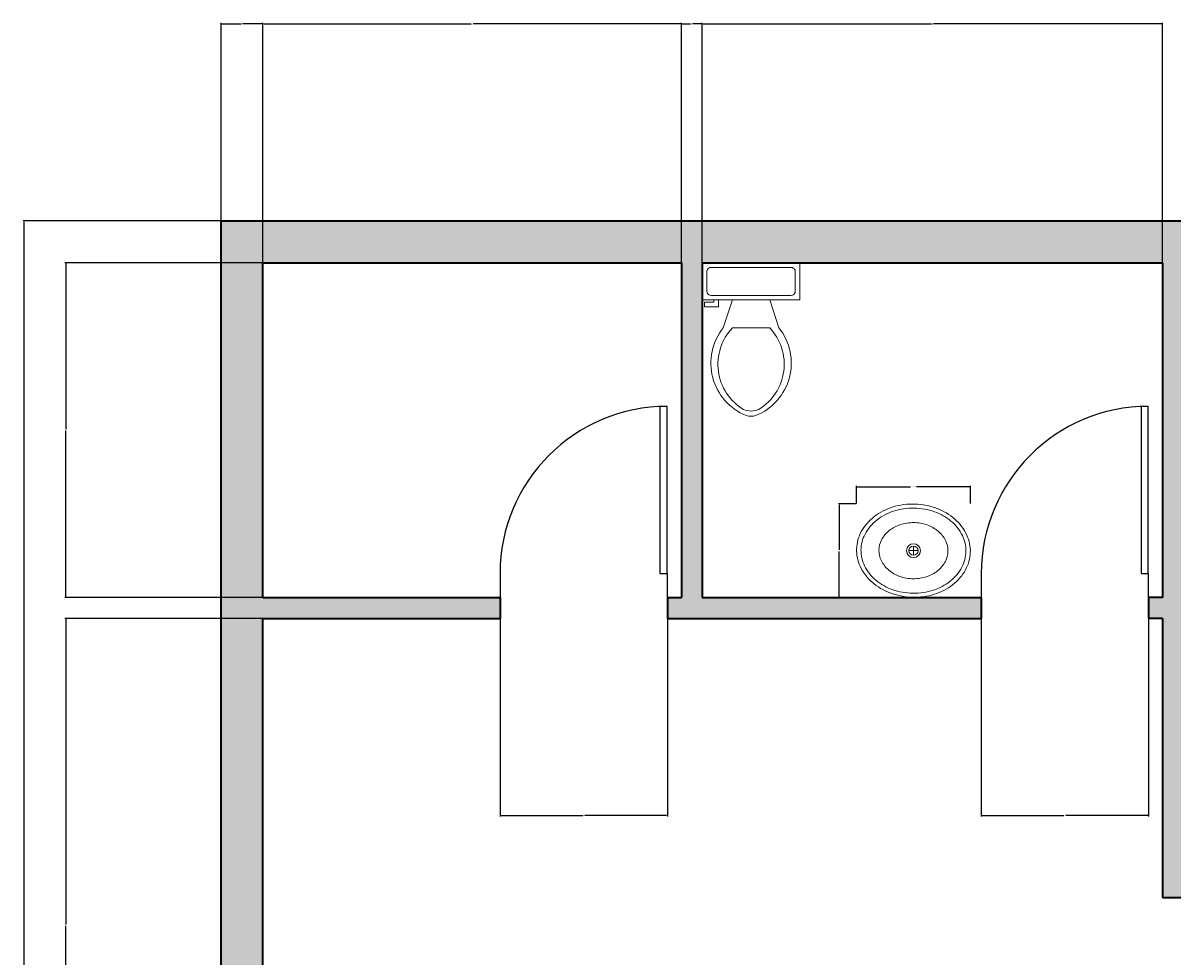
# Model space of a CAD drawing. Units: inches. Extents: x 1563 to 2428, y 777 to 1464.
# Tile 6 of 11: x 1563 to 1810, y 1263 to 1464. Entities that reach past the tile are written whole.
import ezdxf

# ---------------------------------------------------------------- set-up
doc = ezdxf.new("R2010")
doc.units = ezdxf.units.IN
for name, color, linetype, lineweight in [('A-ANNO-DIMS', 2, 'Continuous', 18), ('A-DOOR', 4, 'Continuous', 25), ('A-FLOR-FIXT', 9, 'Continuous', 20), ('A-WALL', 7, 'Continuous', 35), ('A-WALL-PATT', 8, 'Continuous', 13)]:
    doc.layers.add(name, color=color, linetype=linetype, lineweight=lineweight)
doc.styles.get("Standard").update_dxf_attribs({"font": 'arial.ttf'})
doc.dimstyles.get("Standard").update_dxf_attribs({"dimtxt": 0.18, "dimasz": 0.18, "dimexe": 0.18, "dimexo": 0.0625, "dimgap": 0.09, "dimtad": 0, "dimtih": 1, "dimtoh": 1, "dimdec": 4, "dimzin": 0, "dimdsep": 46, "dimtxsty": 'Standard', "dimcen": 0.09, "dimadec": 0, "dimazin": 0, "dimtfac": 1, "dimtdec": 4, "dimtofl": 0, "dimtmove": 0, "dimatfit": 3, "dimfxl": 1, "dimtolj": 1, "dimtzin": 0, "dimarcsym": 0})

# ---------------------------------------------------------------- blocks, each defined once
blk = doc.blocks.new('*U3')
for p, q in [((0, 0), (0, -6)), ((-40, 0), (-40, -6))]:
    blk.add_line(p, q)
blk.add_lwpolyline([(0, 0), (0, 40), (-1.75, 40), (-1.75, 0)], close=True)
blk.add_arc((0, 0), 40, 90, 180)
blk = doc.blocks.new('Toilet - top')
for p, q in [((9.5, -6), (9.5, -2)), ((-10, -8.5), (-8, -8.5)), ((-10, -9.5), (-10, -8.5)), ((-7, -9.5), (-10, -9.5)), ((-8, -8.5), (-8, -8)), ((-7, -8), (-7, -9.5)), ((-4, -8), (-6, -14)), ((4, -8), (6, -14)), ((4, -14), (-4, -14))]:
    blk.add_line(p, q)
blk.add_lwpolyline([(10.5, -8), (10.5, 0), (-10.5, 0), (-10.5, -8)], close=True)
for points in [[(-9.5, -2), (-9.5, -6)], [(8.5, -1), (-8.5, -1)], [(-8.5, -7), (8.5, -7)]]:
    blk.add_lwpolyline(points)
for centre, radius, start, end in [((-8.62, -1.88), 0.884, 81.8699, 188.1301), ((8.62, -1.88), 0.884, 351.8699, 98.1301), ((-8.62, -6.12), 0.884, 171.8699, 278.1301), ((8.62, -6.12), 0.884, 261.8699, 8.1301), ((3.52, -21.58), 12.17, 141.4691, 247.9714), ((4.2, -21.82), 11.33, 136.3677, 238.9468), ((-3.52, -21.58), 12.17, 292.0284, 38.5307), ((-4.2, -21.82), 11.33, 301.053, 43.6321), ((0, -27.88), 4, 245.7318, 294.2682), ((0, -29), 4, 254.8605, 285.1395)]:
    blk.add_arc(centre, radius, start, end)
blk = doc.blocks.new('Sink - Oval top')
for p, q in [((-1, 0), (1, 0)), ((0, 1), (0, -1))]:
    blk.add_line(p, q)
for points in [[(-12.23, 0.39, 0.117634), (-11.46, -3.36, 0.104469), (-8.88, -6.8, 0.090016), (-5.08, -9.07, 0.08192), (-0.32, -10.02, 0.08192), (4.49, -9.38, 0.090016), (8.42, -7.36, 0.104469), (11.22, -4.09, 0.117634), (12.23, -0.39, 0.117634), (11.46, 3.36, 0.104469), (8.88, 6.8, 0.090016), (5.08, 9.07, 0.08192), (0.32, 10.02, 0.08192), (-4.49, 9.38, 0.090016), (-8.42, 7.36, 0.104469), (-11.22, 4.09, 0.117634)], [(-11.29, 0.16, 0.118622), (-10.52, -3.25, 0.104678), (-8.07, -6.36, 0.089562), (-4.54, -8.37, 0.081185), (-0.13, -9.15, 0.081185), (4.3, -8.49, 0.089562), (7.89, -6.58, 0.104678), (10.42, -3.55, 0.118622), (11.29, -0.16, 0.118622), (10.52, 3.25, 0.104678), (8.07, 6.36, 0.089562), (4.54, 8.37, 0.081185), (0.13, 9.15, 0.081185), (-4.3, 8.49, 0.089562), (-7.89, 6.58, 0.104678), (-10.42, 3.55, 0.118622)], [(-7.42, 0.08, 0.118283), (-6.91, -2.17, 0.104607), (-5.29, -4.21, 0.089718), (-2.97, -5.53, 0.081436), (-0.07, -6.04, 0.081436), (2.84, -5.59, 0.089718), (5.2, -4.33, 0.104607), (6.86, -2.32, 0.118283), (7.42, -0.08, 0.118283), (6.91, 2.17, 0.104607), (5.29, 4.21, 0.089718), (2.97, 5.53, 0.081436), (0.07, 6.04, 0.081436), (-2.84, 5.59, 0.089718), (-5.2, 4.33, 0.104607), (-6.86, 2.32, 0.118283)]]:
    blk.add_lwpolyline(points, format="xyb", close=True)
for radius in [1.5, 1]:
    blk.add_circle((0, 0), radius)
blk = doc.blocks.new('*D44')
at = {"layer": 'A-ANNO-DIMS', "color": 0, "lineweight": -2, "transparency": 16777216}
for p, q in [((1741.76, 1360.64), (1741.76, 1364.44)), ((1741.94, 1364.26), (1753.4, 1364.26)), ((1766.13, 1364.26), (1754.66, 1364.26)), ((1766.31, 1360.64), (1766.31, 1364.44))]:
    blk.add_line(p, q, dxfattribs=at)
at = {"layer": 'A-ANNO-DIMS', "color": 0, "transparency": 16777216}
for points in [[(1741.94, 1364.29), (1741.94, 1364.23), (1741.76, 1364.26)], [(1766.13, 1364.29), (1766.13, 1364.23), (1766.31, 1364.26)]]:
    blk.add_solid(points, dxfattribs=at)
at = {"layer": 'Defpoints', "color": 0, "transparency": 16777216}
for p in [(1766.31, 1364.26), (1741.76, 1360.58), (1766.31, 1360.58)]:
    blk.add_point(p, dxfattribs=at)
at = {"layer": 'A-ANNO-DIMS', "color": 0, "transparency": 16777216, "insert": (1754.03, 1364.26), "char_height": 0.18, "attachment_point": 5}
blk.add_mtext('\\A1;BASIN 25', dxfattribs=at)
blk = doc.blocks.new('*D45')
at = {"layer": 'A-ANNO-DIMS', "color": 0, "lineweight": -2, "transparency": 16777216}
for p, q in [((1741.69, 1360.58), (1737.89, 1360.58)), ((1738.07, 1360.4), (1738.07, 1350.69)), ((1738.07, 1340.62), (1738.07, 1350.33)), ((1741.69, 1340.44), (1737.89, 1340.44))]:
    blk.add_line(p, q, dxfattribs=at)
at = {"layer": 'A-ANNO-DIMS', "color": 0, "transparency": 16777216}
for points in [[(1738.04, 1360.4), (1738.1, 1360.4), (1738.07, 1360.58)], [(1738.04, 1340.62), (1738.1, 1340.62), (1738.07, 1340.44)]]:
    blk.add_solid(points, dxfattribs=at)
at = {"layer": 'Defpoints', "color": 0, "transparency": 16777216}
for p in [(1738.07, 1360.58), (1741.76, 1360.58), (1741.76, 1340.44)]:
    blk.add_point(p, dxfattribs=at)
at = {"layer": 'A-ANNO-DIMS', "color": 0, "transparency": 16777216, "insert": (1738.07, 1350.51), "char_height": 0.18, "attachment_point": 5}
blk.add_mtext('\\A1;20', dxfattribs=at)
blk = doc.blocks.new('*D49')
at = {"layer": 'A-ANNO-DIMS', "color": 0, "lineweight": -2, "transparency": 16777216}
for p, q in [((1605.04, 1421.43), (1562.53, 1421.43)), ((1562.71, 1421.25), (1562.71, 1121.61)), ((1562.71, 821.61), (1562.71, 1121.25)), ((1605.04, 821.43), (1562.53, 821.43))]:
    blk.add_line(p, q, dxfattribs=at)
at = {"layer": 'A-ANNO-DIMS', "color": 0, "transparency": 16777216}
for points in [[(1562.68, 1421.25), (1562.74, 1421.25), (1562.71, 1421.43)], [(1562.68, 821.61), (1562.74, 821.61), (1562.71, 821.43)]]:
    blk.add_solid(points, dxfattribs=at)
at = {"layer": 'Defpoints', "color": 0, "transparency": 16777216}
for p in [(1562.71, 1421.43), (1605.11, 1421.43), (1605.11, 821.43)]:
    blk.add_point(p, dxfattribs=at)
at = {"layer": 'A-ANNO-DIMS', "color": 0, "transparency": 16777216, "insert": (1562.71, 1121.43), "char_height": 0.18, "attachment_point": 5}
blk.add_mtext('\\A1;600', dxfattribs=at)
blk = doc.blocks.new('*D50')
at = {"layer": 'A-ANNO-DIMS', "color": 0, "lineweight": -2, "transparency": 16777216}
for p, q in [((1614.11, 1412.49), (1614.11, 1464.01)), ((1614.29, 1463.83), (1658.89, 1463.83)), ((1703.93, 1463.83), (1659.32, 1463.83)), ((1704.11, 1412.49), (1704.11, 1464.01))]:
    blk.add_line(p, q, dxfattribs=at)
at = {"layer": 'A-ANNO-DIMS', "color": 0, "transparency": 16777216}
for points in [[(1614.29, 1463.86), (1614.29, 1463.8), (1614.11, 1463.83)], [(1703.93, 1463.86), (1703.93, 1463.8), (1704.11, 1463.83)]]:
    blk.add_solid(points, dxfattribs=at)
at = {"layer": 'Defpoints', "color": 0, "transparency": 16777216}
for p in [(1704.11, 1463.83), (1614.11, 1412.43), (1704.11, 1412.43)]:
    blk.add_point(p, dxfattribs=at)
at = {"layer": 'A-ANNO-DIMS', "color": 0, "transparency": 16777216, "insert": (1659.11, 1463.83), "char_height": 0.18, "attachment_point": 5}
blk.add_mtext('\\A1;90', dxfattribs=at)
blk = doc.blocks.new('*D51')
at = {"layer": 'A-ANNO-DIMS', "color": 0, "lineweight": -2, "transparency": 16777216}
for p, q in [((1708.61, 1412.49), (1708.61, 1464.01)), ((1708.79, 1463.83), (1757.89, 1463.83)), ((1807.43, 1463.83), (1758.32, 1463.83)), ((1807.61, 1412.49), (1807.61, 1464.01))]:
    blk.add_line(p, q, dxfattribs=at)
at = {"layer": 'A-ANNO-DIMS', "color": 0, "transparency": 16777216}
for points in [[(1708.79, 1463.86), (1708.79, 1463.8), (1708.61, 1463.83)], [(1807.43, 1463.86), (1807.43, 1463.8), (1807.61, 1463.83)]]:
    blk.add_solid(points, dxfattribs=at)
at = {"layer": 'Defpoints', "color": 0, "transparency": 16777216}
for p in [(1807.61, 1463.83), (1708.61, 1412.43), (1807.61, 1412.43)]:
    blk.add_point(p, dxfattribs=at)
at = {"layer": 'A-ANNO-DIMS', "color": 0, "transparency": 16777216, "insert": (1758.11, 1463.83), "char_height": 0.18, "attachment_point": 5}
blk.add_mtext('\\A1;99', dxfattribs=at)
blk = doc.blocks.new('*D53')
at = {"layer": 'A-ANNO-DIMS', "color": 0, "lineweight": -2, "transparency": 16777216}
for p, q in [((1614.04, 1412.43), (1571.53, 1412.43)), ((1571.71, 1412.25), (1571.71, 1376.61)), ((1571.71, 1340.61), (1571.71, 1376.25)), ((1614.04, 1340.43), (1571.53, 1340.43))]:
    blk.add_line(p, q, dxfattribs=at)
at = {"layer": 'A-ANNO-DIMS', "color": 0, "transparency": 16777216}
for points in [[(1571.68, 1412.25), (1571.74, 1412.25), (1571.71, 1412.43)], [(1571.68, 1340.61), (1571.74, 1340.61), (1571.71, 1340.43)]]:
    blk.add_solid(points, dxfattribs=at)
at = {"layer": 'Defpoints', "color": 0, "transparency": 16777216}
for p in [(1571.71, 1412.43), (1614.11, 1412.43), (1614.11, 1340.43)]:
    blk.add_point(p, dxfattribs=at)
at = {"layer": 'A-ANNO-DIMS', "color": 0, "transparency": 16777216, "insert": (1571.71, 1376.43), "char_height": 0.18, "attachment_point": 5}
blk.add_mtext('\\A1;72', dxfattribs=at)
blk = doc.blocks.new('*D55')
at = {"layer": 'A-ANNO-DIMS', "color": 0, "lineweight": -2, "transparency": 16777216}
for p, q in [((1614.04, 1335.93), (1571.53, 1335.93)), ((1571.71, 1335.75), (1571.71, 1270.11)), ((1571.71, 1204.11), (1571.71, 1269.75)), ((1614.04, 1203.93), (1571.53, 1203.93))]:
    blk.add_line(p, q, dxfattribs=at)
at = {"layer": 'A-ANNO-DIMS', "color": 0, "transparency": 16777216}
for points in [[(1571.68, 1335.75), (1571.74, 1335.75), (1571.71, 1335.93)], [(1571.68, 1204.11), (1571.74, 1204.11), (1571.71, 1203.93)]]:
    blk.add_solid(points, dxfattribs=at)
at = {"layer": 'Defpoints', "color": 0, "transparency": 16777216}
for p in [(1571.71, 1335.93), (1614.11, 1335.93), (1614.11, 1203.93)]:
    blk.add_point(p, dxfattribs=at)
at = {"layer": 'A-ANNO-DIMS', "color": 0, "transparency": 16777216, "insert": (1571.71, 1269.93), "char_height": 0.18, "attachment_point": 5}
blk.add_mtext('\\A1;132', dxfattribs=at)
blk = doc.blocks.new('*D65')
at = {"layer": 'A-ANNO-DIMS', "color": 0, "lineweight": -2, "transparency": 16777216}
for p, q in [((1665.11, 1335.87), (1665.11, 1293.35)), ((1701.11, 1335.87), (1701.11, 1293.35)), ((1665.29, 1293.53), (1682.89, 1293.53)), ((1700.93, 1293.53), (1683.32, 1293.53))]:
    blk.add_line(p, q, dxfattribs=at)
at = {"layer": 'A-ANNO-DIMS', "color": 0, "transparency": 16777216}
for points in [[(1665.29, 1293.56), (1665.29, 1293.5), (1665.11, 1293.53)], [(1700.93, 1293.56), (1700.93, 1293.5), (1701.11, 1293.53)]]:
    blk.add_solid(points, dxfattribs=at)
at = {"layer": 'Defpoints', "color": 0, "transparency": 16777216}
for p in [(1665.11, 1335.93), (1701.11, 1335.93), (1665.11, 1293.53)]:
    blk.add_point(p, dxfattribs=at)
at = {"layer": 'A-ANNO-DIMS', "color": 0, "transparency": 16777216, "insert": (1683.11, 1293.53), "char_height": 0.18, "attachment_point": 5}
blk.add_mtext('\\A1;36', dxfattribs=at)
blk = doc.blocks.new('*D66')
at = {"layer": 'A-ANNO-DIMS', "color": 0, "lineweight": -2, "transparency": 16777216}
for p, q in [((1768.61, 1335.87), (1768.61, 1293.35)), ((1804.61, 1335.87), (1804.61, 1293.35)), ((1768.79, 1293.53), (1786.39, 1293.53)), ((1804.43, 1293.53), (1786.82, 1293.53))]:
    blk.add_line(p, q, dxfattribs=at)
at = {"layer": 'A-ANNO-DIMS', "color": 0, "transparency": 16777216}
for points in [[(1768.79, 1293.56), (1768.79, 1293.5), (1768.61, 1293.53)], [(1804.43, 1293.56), (1804.43, 1293.5), (1804.61, 1293.53)]]:
    blk.add_solid(points, dxfattribs=at)
at = {"layer": 'Defpoints', "color": 0, "transparency": 16777216}
for p in [(1768.61, 1335.93), (1804.61, 1335.93), (1768.61, 1293.53)]:
    blk.add_point(p, dxfattribs=at)
at = {"layer": 'A-ANNO-DIMS', "color": 0, "transparency": 16777216, "insert": (1786.61, 1293.53), "char_height": 0.18, "attachment_point": 5}
blk.add_mtext('\\A1;36', dxfattribs=at)
blk = doc.blocks.new('*D71')
at = {"layer": 'A-ANNO-DIMS', "color": 0, "lineweight": -2, "transparency": 16777216}
for p, q in [((1704.11, 1412.49), (1704.11, 1464.01)), ((1704.29, 1463.83), (1706.1, 1463.83)), ((1708.43, 1463.83), (1706.61, 1463.83)), ((1708.61, 1412.49), (1708.61, 1464.01))]:
    blk.add_line(p, q, dxfattribs=at)
at = {"layer": 'A-ANNO-DIMS', "color": 0, "transparency": 16777216}
for points in [[(1704.29, 1463.86), (1704.29, 1463.8), (1704.11, 1463.83)], [(1708.43, 1463.86), (1708.43, 1463.8), (1708.61, 1463.83)]]:
    blk.add_solid(points, dxfattribs=at)
at = {"layer": 'Defpoints', "color": 0, "transparency": 16777216}
for p in [(1708.61, 1463.83), (1704.11, 1412.43), (1708.61, 1412.43)]:
    blk.add_point(p, dxfattribs=at)
at = {"layer": 'A-ANNO-DIMS', "color": 0, "transparency": 16777216, "insert": (1706.36, 1463.83), "char_height": 0.18, "attachment_point": 5}
blk.add_mtext('\\A1;4.5', dxfattribs=at)
blk = doc.blocks.new('*D72')
at = {"layer": 'A-ANNO-DIMS', "color": 0, "lineweight": -2, "transparency": 16777216}
for p, q in [((1605.11, 1421.49), (1605.11, 1464.01)), ((1605.29, 1463.83), (1609.46, 1463.83)), ((1613.93, 1463.83), (1609.75, 1463.83)), ((1614.11, 1412.49), (1614.11, 1464.01))]:
    blk.add_line(p, q, dxfattribs=at)
at = {"layer": 'A-ANNO-DIMS', "color": 0, "transparency": 16777216}
for points in [[(1605.29, 1463.86), (1605.29, 1463.8), (1605.11, 1463.83)], [(1613.93, 1463.86), (1613.93, 1463.8), (1614.11, 1463.83)]]:
    blk.add_solid(points, dxfattribs=at)
at = {"layer": 'Defpoints', "color": 0, "transparency": 16777216}
for p in [(1614.11, 1463.83), (1605.11, 1421.43), (1614.11, 1412.43)]:
    blk.add_point(p, dxfattribs=at)
at = {"layer": 'A-ANNO-DIMS', "color": 0, "transparency": 16777216, "insert": (1609.61, 1463.83), "char_height": 0.18, "attachment_point": 5}
blk.add_mtext('\\A1;9', dxfattribs=at)

msp = doc.modelspace()

# ---------------------------------------------------------------- hatches: boundary and pattern name
at = {"layer": 'A-WALL-PATT'}
h = msp.add_hatch(color=256, dxfattribs=at)
h.dxf.hatch_style = 1
h.paths.add_polyline_path([(1965.105, 1421.428), (1605.105, 1421.428), (1605.105, 821.428), (1965.105, 821.428)])
h.paths.add_polyline_path([(1614.105, 1199.428), (1704.105, 1199.428), (1738.605, 1199.428), (1738.605, 1251.928), (1734.105, 1251.928), (1734.105, 1203.928), (1704.105, 1203.928), (1614.105, 1203.928), (1614.105, 1335.928), (1665.105, 1335.928), (1665.105, 1340.428), (1614.105, 1340.428), (1614.105, 1412.428), (1704.105, 1412.428), (1704.105, 1340.428), (1701.105, 1340.428), (1701.105, 1335.928), (1704.105, 1335.928), (1768.605, 1335.928), (1768.605, 1340.428), (1708.605, 1340.428), (1708.605, 1412.428), (1807.605, 1412.428), (1807.605, 1340.428), (1804.605, 1340.428), (1804.605, 1335.928), (1807.605, 1335.928), (1807.605, 1275.928), (1815.105, 1275.928), (1815.105, 1280.428), (1812.105, 1280.428), (1812.105, 1412.428), (1956.105, 1412.428), (1956.105, 1280.428), (1854.105, 1280.428), (1854.105, 1275.928), (1956.105, 1275.928), (1956.105, 830.428), (1614.105, 830.428)], flags=16)
h.paths.add_polyline_path([(1917.224, 1038.928), (1917.224, 1043.846, -0.4014527), (1951.591, 1079.751), (1951.591, 1079.786), (1953.163, 1079.786), (1953.163, 1043.846), (1953.163, 1038.455), (1953.105, 1034.428), (1953.105, 1038.928), (1953.163, 1043.846), (1951.591, 1043.846), (1951.591, 1079.751, 0.4014527), (1917.224, 1043.846), (1917.224, 1038.455), (1917.224, 1034.428), (1834.605, 1034.428), (1834.605, 906.928), (1858.605, 906.928), (1858.605, 954.928), (1932.105, 954.928), (1932.105, 902.428), (1834.605, 902.428), (1834.605, 1034.428), (1914.224, 1034.428), (1914.224, 1038.928)], flags=0)
edge = h.paths.add_edge_path(flags=0)
edge.add_ellipse((1674.345, 1004.483), major_axis=(1.48, 0), ratio=0.8423039, start_angle=90, end_angle=180, ccw=False)
edge.add_line((1674.345, 1005.73), (1674.921, 1005.73))
edge.add_ellipse((2202.617, 985.642), major_axis=(528.234, 0), ratio=0.8423039, start_angle=176.34957, end_angle=177.82005, ccw=False)
edge.add_ellipse((1739.278, 760.804), major_axis=(-313.308, 0), ratio=0.8423039, start_angle=-77.87403, end_angle=-76.21947, ccw=False)
edge.add_ellipse((1739.278, 767.659), major_axis=(305.303, 0), ratio=0.8423039, start_angle=100.20954, end_angle=102.44463, ccw=False)
edge.add_ellipse((1659.357, 1231.328), major_axis=(250.96, 0), ratio=0.8423039, start_angle=-80.74343, end_angle=-77.44507)
edge.add_line((1705.625, 1023.567), (1711.685, 1026.918))
edge.add_ellipse((1711.754, 1026.21), major_axis=(0.74, 0), ratio=0.8423039, start_angle=52.06687, end_angle=90, ccw=False)
edge.add_line((1712.16, 1026.731), (1717.882, 1023.567))
edge.add_ellipse((1764.151, 1231.328), major_axis=(250.96, 0), ratio=0.8423039, start_angle=257.44507, end_angle=260.74343)
edge.add_ellipse((1684.229, 767.659), major_axis=(305.303, 0), ratio=0.8423039, start_angle=77.55537, end_angle=79.79046, ccw=False)
edge.add_ellipse((1684.229, 760.804), major_axis=(-313.308, 0), ratio=0.8423039, start_angle=256.21947, end_angle=257.87403, ccw=False)
edge.add_ellipse((1220.891, 985.642), major_axis=(-528.234, 0), ratio=0.8423039, start_angle=182.17995, end_angle=183.65043, ccw=False)
edge.add_line((1748.586, 1005.73), (1749.162, 1005.73))
edge.add_ellipse((1749.162, 1004.483), major_axis=(-1.48, 0), ratio=0.8423039, start_angle=180, end_angle=270, ccw=False)
edge.add_line((1750.642, 1004.483), (1750.642, 980.28))
edge.add_ellipse((1749.162, 980.28), major_axis=(1.48, 0), ratio=0.8423039, start_angle=270, end_angle=360, ccw=False)
edge.add_ellipse((-8843.864, 962.352), major_axis=(10593.026, 0), ratio=0.84230387, start_angle=-0.3241203, end_angle=0.0902291, ccw=False)
edge.add_ellipse((-8843.864, 962.352), major_axis=(10593.026, 0), ratio=0.84230387, start_angle=-0.3838668, end_angle=-0.3241203, ccw=False)
edge.add_ellipse((1749.162, 890.136), major_axis=(1.48, 0), ratio=0.8423039, start_angle=0, end_angle=90, ccw=False)
edge.add_line((1750.642, 890.136), (1750.642, 865.933))
edge.add_ellipse((1749.162, 865.933), major_axis=(1.48, 0), ratio=0.8423039, start_angle=270, end_angle=360, ccw=False)
edge.add_line((1749.162, 864.686), (1748.528, 864.686))
edge.add_ellipse((-8843.864, 962.352), major_axis=(10593.026, 0), ratio=0.84230387, start_angle=-0.6186432, end_angle=-0.5282715, ccw=False)
edge.add_ellipse((1747.592, 846.206), major_axis=(-2.22, 0), ratio=0.8423039, start_angle=179.37176, end_angle=248.46476, ccw=False)
edge.add_ellipse((-8844.604, 962.352), major_axis=(-10595.313, 0), ratio=0.842303864, start_angle=179.3534459, end_angle=179.3717628, ccw=False)
edge.add_ellipse((1744.512, 842.854), major_axis=(-5.246, 0), ratio=0.8423039, start_angle=90, end_angle=179.35345, ccw=False)
edge.add_line((1744.512, 838.435), (1678.995, 838.435))
edge.add_ellipse((1678.995, 842.854), major_axis=(5.246, 0), ratio=0.8423039, start_angle=180.64655, end_angle=270, ccw=False)
edge.add_ellipse((12268.111, 962.352), major_axis=(-10595.313, 0), ratio=0.84230387, start_angle=0.6282372, end_angle=0.6465541, ccw=False)
edge.add_ellipse((1675.916, 846.206), major_axis=(-2.22, 0), ratio=0.8423039, start_angle=-68.46476, end_angle=0.62824, ccw=False)
edge.add_ellipse((12267.371, 962.352), major_axis=(-10593.026, 0), ratio=0.84230387, start_angle=0.5282715, end_angle=0.6465541, ccw=False)
edge.add_line((1674.98, 864.686), (1674.345, 864.686))
edge.add_ellipse((1674.345, 865.933), major_axis=(-1.48, 0), ratio=0.8423039, start_angle=0, end_angle=90, ccw=False)
edge.add_line((1672.865, 865.933), (1672.865, 890.136))
edge.add_ellipse((1674.345, 890.136), major_axis=(1.48, 0), ratio=0.8423039, start_angle=90, end_angle=180, ccw=False)
edge.add_ellipse((12267.371, 962.352), major_axis=(-10593.026, 0), ratio=0.84230387, start_angle=0.3241203, end_angle=0.3838668, ccw=False)
edge.add_ellipse((12267.371, 962.352), major_axis=(-10593.026, 0), ratio=0.84230387, start_angle=-0.0902291, end_angle=0.3241203, ccw=False)
edge.add_ellipse((1674.345, 980.28), major_axis=(-1.48, 0), ratio=0.8423039, start_angle=0, end_angle=90, ccw=False)
edge.add_line((1672.865, 980.28), (1672.865, 1004.483))
h.paths.add_polyline_path([(1622.542, 1135.584), (1648.534, 1136.233), (1648.683, 1130.234), (1647.126, 1130.196), (1648.323, 1082.21), (1649.88, 1082.249), (1650.03, 1076.251), (1624.038, 1075.603, -0.266667)], flags=0)
edge = h.paths.add_edge_path(flags=0)
edge.add_line((1694.584, 990.705), (1700.334, 994.711))
edge.add_line((1700.334, 994.711), (1702.248, 994.711))
edge.add_line((1702.248, 994.711), (1702.248, 997.061))
edge.add_ellipse((1758.417, 997.061), major_axis=(56.169, 0), ratio=0.8423039, start_angle=150.56143, end_angle=180, ccw=False)
edge.add_ellipse((1665.091, 997.061), major_axis=(-56.169, 0), ratio=0.8423039, start_angle=180, end_angle=209.43857, ccw=False)
edge.add_line((1721.26, 997.061), (1721.26, 994.711))
edge.add_line((1721.26, 994.711), (1723.174, 994.711))
edge.add_line((1723.174, 994.711), (1728.923, 990.705))
edge.add_line((1728.923, 990.705), (1728.923, 975.895))
edge.add_ellipse((1725.091, 976.043), major_axis=(0.357, 6.34), ratio=0.6038336, start_angle=106.34259, end_angle=270.99799, ccw=False)
edge.add_line((1721.26, 975.15), (1721.26, 997.061))
edge.add_ellipse((1665.091, 997.061), major_axis=(-56.169, 0), ratio=0.8423039, start_angle=180, end_angle=209.43857)
edge.add_ellipse((1758.417, 997.061), major_axis=(56.169, 0), ratio=0.8423039, start_angle=150.56143, end_angle=180)
edge.add_line((1702.248, 997.061), (1702.248, 975.15))
edge.add_ellipse((1698.416, 976.043), major_axis=(-0.357, 6.34), ratio=0.6038336, start_angle=89.00201, end_angle=253.65741, ccw=False)
edge.add_line((1694.584, 975.895), (1694.584, 990.705))
edge = h.paths.add_edge_path(flags=0)
edge.add_line((1675.832, 952.075), (1679.883, 938.848))
edge.add_ellipse((5378.107, 931.045), major_axis=(-3698.236, 0), ratio=0.84230387, start_angle=-0.120897, end_angle=0.364076)
edge.add_line((1679.976, 907.545), (1676.149, 892.52))
edge.add_ellipse((12267.371, 962.352), major_axis=(10591.546, 0), ratio=0.84230387, start_angle=180.3241656, end_angle=180.3777642, ccw=False)
edge.add_ellipse((12267.371, 962.352), major_axis=(10591.546, 0), ratio=0.84230387, start_angle=180.0555943, end_angle=180.3241656, ccw=False)
edge = h.paths.add_edge_path(flags=0)
edge.add_ellipse((1706.366, 891.542), major_axis=(81.773, 0), ratio=0.8423039, start_angle=94.27742, end_angle=111.83495, ccw=False)
edge.add_line((1701.225, 960.283), (1722.283, 960.283))
edge.add_ellipse((1717.141, 891.542), major_axis=(-81.773, 0), ratio=0.8423039, start_angle=248.16505, end_angle=265.72258, ccw=False)
edge.add_line((1743.29, 956.803), (1741.105, 940.427))
edge.add_ellipse((1714.553, 877.238), major_axis=(79.58, 0), ratio=0.8423039, start_angle=67.20809, end_angle=85.12993)
edge.add_line((1720.25, 944.097), (1703.258, 944.097))
edge.add_ellipse((1708.954, 877.238), major_axis=(79.58, 0), ratio=0.8423039, start_angle=94.87007, end_angle=112.79191)
edge.add_line((1682.403, 940.427), (1680.218, 956.803))
h.paths.add_polyline_path([(1664.992, 1093.991), (1664.992, 1123.991), (1724.992, 1123.991), (1724.992, 1093.991)], flags=0)
h.paths.add_polyline_path([(1716.588, 1099.729), (1715.404, 1099.805), (1715.021, 1099.823), (1716.177, 1099.758)], flags=0)
h.paths.add_polyline_path([(1711.325, 1103.757), (1712.167, 1103.706), (1713.009, 1103.642), (1713.84, 1103.566), (1715.041, 1103.439), (1716.532, 1103.244), (1717.793, 1103.048), (1718.876, 1102.854), (1719.676, 1102.699), (1720.157, 1102.605), (1720.632, 1102.513), (1721.109, 1102.424), (1721.595, 1102.339), (1722.088, 1102.264), (1722.585, 1102.205), (1723.082, 1102.17), (1723.575, 1102.164), (1724.321, 1102.211), (1724.533, 1102.268), (1723.842, 1102.16), (1722.864, 1102.172), (1721.894, 1102.287), (1720.935, 1102.454), (1720.157, 1102.605), (1719.676, 1102.699), (1719.18, 1102.795), (1718.66, 1102.892), (1718.109, 1102.991), (1717.517, 1103.091), (1716.876, 1103.191), (1716.179, 1103.29), (1715.435, 1103.387), (1714.652, 1103.48), (1713.84, 1103.566), (1713.009, 1103.642), (1712.167, 1103.706), (1711.325, 1103.757), (1710.492, 1103.791), (1709.676, 1103.806), (1708.873, 1103.805), (1707.707, 1103.78), (1707.292, 1103.757), (1708.499, 1103.805), (1710.086, 1103.807)], flags=0)
h.paths.add_polyline_path([(1713.959, 1106.591), (1714.651, 1106.624), (1715.279, 1106.674), (1715.852, 1106.736), (1716.373, 1106.807), (1716.851, 1106.885), (1717.289, 1106.966), (1717.696, 1107.046), (1718.341, 1107.178), (1719.173, 1107.331), (1720.169, 1107.421), (1721.131, 1107.383), (1722.032, 1107.286), (1722.934, 1107.152), (1723.887, 1106.983), (1724.746, 1106.795), (1724.72, 1106.798), (1724.663, 1106.807), (1724.241, 1106.906), (1724.159, 1106.924), (1723.885, 1106.979), (1723.546, 1107.044), (1723.157, 1107.113), (1722.732, 1107.182), (1722.284, 1107.249), (1721.827, 1107.308), (1721.375, 1107.357), (1720.942, 1107.391), (1720.539, 1107.406), (1720.162, 1107.405), (1719.804, 1107.388), (1719.459, 1107.357), (1719.12, 1107.314), (1718.781, 1107.259), (1718.435, 1107.195), (1718.076, 1107.124), (1717.402, 1106.986), (1716.59, 1106.837), (1715.56, 1106.696), (1714.317, 1106.598)], flags=0)
h.paths.add_polyline_path([(1708.692, 1110.124), (1709.455, 1110.13), (1710.147, 1110.149), (1710.772, 1110.18), (1711.334, 1110.224), (1711.836, 1110.28), (1712.283, 1110.349), (1712.678, 1110.43), (1713.026, 1110.524), (1713.33, 1110.63), (1713.596, 1110.746), (1713.832, 1110.87), (1714.042, 1110.999), (1714.234, 1111.131), (1714.413, 1111.264), (1714.586, 1111.396), (1715.065, 1111.75), (1715.879, 1112.11), (1716.842, 1112.224), (1717.903, 1112.165), (1719.048, 1111.965), (1719.867, 1111.736), (1720.686, 1111.487), (1721.596, 1111.22), (1721.917, 1111.136), (1721.028, 1111.383), (1720.222, 1111.628), (1719.815, 1111.75), (1719.434, 1111.857), (1719.054, 1111.951), (1718.672, 1112.031), (1718.292, 1112.097), (1717.918, 1112.149), (1717.554, 1112.185), (1717.204, 1112.204), (1716.871, 1112.206), (1716.559, 1112.191), (1716.271, 1112.156), (1716.006, 1112.105), (1715.761, 1112.038), (1715.534, 1111.957), (1715.323, 1111.864), (1715.125, 1111.759), (1714.937, 1111.645), (1714.759, 1111.524), (1714.586, 1111.396), (1714.413, 1111.264), (1714.003, 1110.96), (1713.331, 1110.606), (1712.501, 1110.382), (1711.61, 1110.245), (1710.489, 1110.158), (1709.111, 1110.121)], flags=0)
h.paths.add_polyline_path([(1707.127, 1113.075), (1707.639, 1113.025), (1708.092, 1112.991), (1708.49, 1112.975), (1708.836, 1112.977), (1709.135, 1112.996), (1709.392, 1113.032), (1709.612, 1113.084), (1709.798, 1113.15), (1709.957, 1113.23), (1710.092, 1113.324), (1710.208, 1113.431), (1710.304, 1113.554), (1710.379, 1113.698), (1710.434, 1113.866), (1710.467, 1114.062), (1710.477, 1114.289), (1710.463, 1114.553), (1710.426, 1114.857), (1710.364, 1115.202), (1710.282, 1115.58), (1710.184, 1115.98), (1710.076, 1116.391), (1709.961, 1116.801), (1709.844, 1117.201), (1709.731, 1117.579), (1709.626, 1117.924), (1709.532, 1118.228), (1709.454, 1118.493), (1709.392, 1118.723), (1709.351, 1118.924), (1709.293, 1119.435), (1709.831, 1119.942), (1710.705, 1120.121), (1711.507, 1119.898), (1712.224, 1119.567), (1713.189, 1119.016), (1713.529, 1118.804), (1712.958, 1119.148), (1712.468, 1119.428), (1712.046, 1119.649), (1711.683, 1119.817), (1711.366, 1119.937), (1711.084, 1120.016), (1710.826, 1120.057), (1710.582, 1120.067), (1710.354, 1120.049), (1710.142, 1120.006), (1709.951, 1119.941), (1709.781, 1119.857), (1709.635, 1119.757), (1709.516, 1119.645), (1709.426, 1119.524), (1709.366, 1119.395), (1709.335, 1119.255), (1709.331, 1119.1), (1709.351, 1118.924), (1709.392, 1118.723), (1709.454, 1118.493), (1709.52, 1118.268), (1709.799, 1117.356), (1710.028, 1116.57), (1710.245, 1115.749), (1710.45, 1114.804), (1710.477, 1114.289), (1710.448, 1113.654), (1709.908, 1113.153), (1709.165, 1112.979), (1708.318, 1112.974), (1707.448, 1113.039)], flags=0)
h.paths.add_polyline_path([(1700.892, 1119.857), (1701.604, 1119.819), (1702.196, 1119.805), (1702.683, 1119.813), (1703.076, 1119.841), (1703.387, 1119.887), (1703.63, 1119.951), (1703.816, 1120.03), (1703.959, 1120.124), (1704.069, 1120.23), (1704.15, 1120.346), (1704.204, 1120.47), (1704.234, 1120.599), (1704.242, 1120.731), (1704.231, 1120.864), (1704.202, 1120.996), (1704.159, 1121.124), (1704.103, 1121.246), (1704.039, 1121.362), (1703.97, 1121.474), (1703.901, 1121.582), (1703.834, 1121.687), (1703.775, 1121.79), (1703.564, 1122.226), (1704.048, 1122.698), (1704.756, 1122.769), (1705.49, 1122.723), (1706.24, 1122.641), (1706.547, 1122.601), (1706.092, 1122.657), (1705.695, 1122.701), (1705.348, 1122.732), (1705.049, 1122.751), (1704.792, 1122.757), (1704.573, 1122.751), (1704.386, 1122.732), (1704.227, 1122.701), (1704.092, 1122.657), (1703.977, 1122.601), (1703.88, 1122.534), (1703.802, 1122.458), (1703.742, 1122.374), (1703.702, 1122.284), (1703.68, 1122.188), (1703.677, 1122.09), (1703.692, 1121.991), (1703.726, 1121.89), (1703.769, 1121.802), (1704.039, 1121.362), (1704.301, 1120.887), (1704.133, 1120.165), (1703.43, 1119.866), (1702.481, 1119.798), (1701.306, 1119.827)], flags=0)
edge = h.paths.add_edge_path(flags=0)
edge.add_ellipse((1711.754, 1009.752), major_axis=(-147.018, 0), ratio=0.8423039, start_angle=76.40187, end_angle=103.59813)
edge.add_line((1741.105, 888.411), (1741.105, 869.587))
edge.add_ellipse((1711.754, 990.928), major_axis=(-147.018, 0), ratio=0.8423039, start_angle=76.40187, end_angle=103.59813, ccw=False)
edge.add_line((1682.403, 869.587), (1682.403, 888.411))
edge = h.paths.add_edge_path(flags=0)
edge.add_ellipse((-8843.864, 962.352), major_axis=(-10591.546, 0), ratio=0.84230387, start_angle=179.6758344, end_angle=179.9444057, ccw=False)
edge.add_ellipse((-8843.864, 962.352), major_axis=(-10591.546, 0), ratio=0.84230387, start_angle=179.6222358, end_angle=179.6758344, ccw=False)
edge.add_line((1747.358, 892.52), (1743.531, 907.545))
edge.add_ellipse((-1954.6, 931.045), major_axis=(3698.236, 0), ratio=0.84230387, start_angle=-0.364076, end_angle=0.120897)
edge.add_line((1743.625, 938.848), (1747.676, 952.075))
h.paths.add_polyline_path([(1637.931, 1162.087), (1637.931, 1188.087, -0.1904762), (1721.931, 1188.087), (1721.931, 1162.087), (1715.931, 1162.087), (1715.931, 1163.644), (1643.931, 1163.644), (1643.931, 1162.087)], flags=0)
h.paths.add_polyline_path([(1667.931, 1189.491, -0.0496282), (1691.931, 1189.491), (1691.931, 1182.705), (1667.931, 1182.705)], flags=0)
edge = h.paths.add_edge_path(flags=0)
edge.add_ellipse((1685.362, 859.825), major_axis=(-2.96, 0), ratio=0.8423039, start_angle=-90, end_angle=0, ccw=False)
edge.add_line((1685.362, 862.318), (1738.145, 862.318))
edge.add_ellipse((1738.145, 859.825), major_axis=(2.96, 0), ratio=0.8423039, start_angle=0, end_angle=90, ccw=False)
edge.add_line((1741.105, 859.825), (1741.105, 840.361))
edge.add_line((1741.105, 840.361), (1682.403, 840.361))
edge.add_line((1682.403, 840.361), (1682.403, 859.825))
h.paths.add_polyline_path([(1777.486, 1164.853), (1777.486, 1180.853), (1778.486, 1181.01), (1778.486, 1164.697)], flags=0)
h.paths.add_polyline_path([(1786.986, 1154.853), (1786.986, 1163.369), (1778.986, 1164.619), (1778.986, 1181.088), (1786.986, 1182.338), (1786.986, 1190.853), (1799.502, 1190.853), (1800.752, 1198.853), (1817.221, 1198.853), (1818.471, 1190.853), (1827.502, 1190.853), (1828.752, 1198.853), (1845.221, 1198.853), (1846.471, 1190.853), (1858.986, 1190.853), (1858.986, 1182.338), (1866.986, 1181.088), (1866.986, 1164.619), (1858.986, 1163.369), (1858.986, 1154.853), (1846.471, 1154.853), (1845.221, 1146.853), (1828.752, 1146.853), (1827.502, 1154.853), (1818.471, 1154.853), (1817.221, 1146.853), (1800.752, 1146.853), (1799.502, 1154.853)], flags=0)
h.paths.add_polyline_path([(1800.986, 1145.353), (1800.83, 1146.353), (1817.143, 1146.353), (1816.986, 1145.353)], flags=0)
h.paths.add_polyline_path([(1851.408, 1167.858), (1852.086, 1167.738), (1852.744, 1167.621), (1853.388, 1167.506), (1854.028, 1167.395), (1854.67, 1167.289), (1855.313, 1167.195), (1855.952, 1167.122), (1856.585, 1167.077), (1857.209, 1167.07), (1858.147, 1167.128), (1858.413, 1167.2), (1857.547, 1167.066), (1856.312, 1167.08), (1855.07, 1167.223), (1854.028, 1167.395), (1853.388, 1167.506), (1852.744, 1167.621), (1852.086, 1167.738), (1851.408, 1167.858), (1850.288, 1168.052), (1849.956, 1168.104), (1850.701, 1167.98)], flags=0)
h.paths.add_polyline_path([(1845.435, 1172.646), (1846.222, 1172.707), (1846.941, 1172.785), (1847.601, 1172.874), (1848.21, 1172.971), (1848.777, 1173.072), (1849.311, 1173.173), (1850.14, 1173.331), (1851.063, 1173.483), (1852.014, 1173.591), (1853.012, 1173.633), (1854.075, 1173.594), (1855.251, 1173.473), (1856.4, 1173.306), (1857.391, 1173.132), (1857.945, 1173.02), (1858.196, 1172.965), (1858.595, 1172.871), (1858.575, 1172.874), (1858.49, 1172.894), (1858.371, 1172.924), (1858.196, 1172.965), (1857.945, 1173.02), (1857.602, 1173.089), (1857.177, 1173.17), (1856.687, 1173.256), (1856.148, 1173.343), (1855.575, 1173.426), (1854.986, 1173.5), (1854.395, 1173.561), (1853.82, 1173.603), (1853.272, 1173.623), (1852.749, 1173.622), (1852.247, 1173.6), (1851.757, 1173.562), (1851.276, 1173.507), (1850.796, 1173.439), (1850.313, 1173.359), (1849.82, 1173.27), (1849.311, 1173.173), (1848.421, 1173.005), (1847.25, 1172.818), (1845.826, 1172.665)], flags=0)
h.paths.add_polyline_path([(1840.587, 1177.09), (1841.289, 1177.145), (1841.916, 1177.215), (1842.475, 1177.301), (1842.969, 1177.403), (1843.403, 1177.52), (1843.783, 1177.652), (1844.117, 1177.797), (1844.411, 1177.952), (1844.674, 1178.114), (1844.914, 1178.279), (1845.138, 1178.446), (1845.644, 1178.831), (1846.285, 1179.221), (1847.125, 1179.521), (1847.998, 1179.624), (1848.834, 1179.619), (1849.768, 1179.529), (1850.775, 1179.363), (1851.78, 1179.14), (1852.111, 1179.053), (1851.57, 1179.187), (1851.043, 1179.304), (1850.527, 1179.404), (1850.024, 1179.487), (1849.539, 1179.551), (1849.072, 1179.596), (1848.628, 1179.62), (1848.21, 1179.623), (1847.82, 1179.603), (1847.46, 1179.561), (1847.128, 1179.497), (1846.822, 1179.413), (1846.539, 1179.312), (1846.274, 1179.195), (1846.027, 1179.064), (1845.793, 1178.922), (1845.57, 1178.77), (1845.354, 1178.61), (1844.817, 1178.201), (1844.106, 1177.764), (1843.208, 1177.452), (1842.225, 1177.25), (1840.973, 1177.11)], flags=0)
h.paths.add_polyline_path([(1836.67, 1180.646), (1837.236, 1180.603), (1837.734, 1180.584), (1838.166, 1180.586), (1838.54, 1180.611), (1838.861, 1180.655), (1839.136, 1180.72), (1839.369, 1180.803), (1839.568, 1180.903), (1839.736, 1181.02), (1839.881, 1181.152), (1840.001, 1181.299), (1840.095, 1181.456), (1840.164, 1181.624), (1840.204, 1181.8), (1840.217, 1181.981), (1840.2, 1182.166), (1840.153, 1182.353), (1840.076, 1182.541), (1839.973, 1182.728), (1839.851, 1182.916), (1839.716, 1183.103), (1839.572, 1183.291), (1839.427, 1183.478), (1839.033, 1184), (1838.862, 1184.411), (1838.695, 1184.99), (1839.2, 1185.669), (1840.06, 1185.961), (1840.793, 1185.931), (1841.454, 1185.77), (1842.179, 1185.536), (1842.706, 1185.363), (1843.713, 1185.044), (1844.033, 1184.956), (1843.102, 1185.234), (1842.179, 1185.536), (1841.725, 1185.682), (1841.328, 1185.801), (1840.976, 1185.886), (1840.653, 1185.937), (1840.349, 1185.949), (1840.063, 1185.926), (1839.799, 1185.872), (1839.559, 1185.791), (1839.347, 1185.686), (1839.165, 1185.562), (1839.016, 1185.422), (1838.903, 1185.27), (1838.828, 1185.11), (1838.79, 1184.943), (1838.784, 1184.77), (1838.809, 1184.593), (1838.862, 1184.411), (1838.938, 1184.227), (1839.036, 1184.041), (1839.153, 1183.853), (1839.285, 1183.666), (1839.427, 1183.478), (1839.572, 1183.291), (1839.716, 1183.103), (1839.851, 1182.916), (1840.178, 1182.415), (1840.251, 1181.604), (1839.686, 1180.915), (1838.893, 1180.633), (1837.976, 1180.574), (1837.01, 1180.612)], flags=0)
h.paths.add_polyline_path([(1829.867, 1185.622), (1830.475, 1185.631), (1830.966, 1185.666), (1831.355, 1185.724), (1831.658, 1185.804), (1831.891, 1185.903), (1832.07, 1186.02), (1832.207, 1186.152), (1832.308, 1186.297), (1832.376, 1186.452), (1832.414, 1186.614), (1832.424, 1186.779), (1832.41, 1186.946), (1832.374, 1187.11), (1832.32, 1187.27), (1832.25, 1187.422), (1832.17, 1187.568), (1832.084, 1187.708), (1831.997, 1187.843), (1831.914, 1187.974), (1831.839, 1188.102), (1831.614, 1188.57), (1832.036, 1189.169), (1832.801, 1189.319), (1833.589, 1189.3), (1834.44, 1189.223), (1834.736, 1189.187), (1834.239, 1189.241), (1833.807, 1189.28), (1833.433, 1189.304), (1833.111, 1189.312), (1832.837, 1189.304), (1832.604, 1189.28), (1832.405, 1189.241), (1832.236, 1189.187), (1832.092, 1189.117), (1831.971, 1189.033), (1831.873, 1188.938), (1831.799, 1188.832), (1831.748, 1188.719), (1831.721, 1188.601), (1831.717, 1188.478), (1831.736, 1188.353), (1831.779, 1188.228), (1831.839, 1188.102), (1831.914, 1187.974), (1831.997, 1187.843), (1832.084, 1187.708), (1832.387, 1187.216), (1832.456, 1186.393), (1831.916, 1185.871), (1831.195, 1185.682), (1830.221, 1185.613)], flags=0)
h.paths.add_polyline_path([(1828.986, 1145.353), (1828.83, 1146.353), (1845.143, 1146.353), (1844.986, 1145.353)], flags=0)
h.paths.add_polyline_path([(1800.986, 1200.353), (1816.986, 1200.353), (1817.143, 1199.353), (1800.83, 1199.353)], flags=0)
h.paths.add_polyline_path([(1828.986, 1200.353), (1844.986, 1200.353), (1845.143, 1199.353), (1828.83, 1199.353)], flags=0)
h.paths.add_polyline_path([(1867.486, 1181.01), (1868.486, 1180.853), (1868.486, 1164.853), (1867.486, 1164.697)], flags=0)
h.paths.add_polyline_path([(1901.055, 1112.089), (1901.055, 1241.889), (1954.299, 1241.889), (1954.299, 1112.089)], flags=0)
h.paths.add_polyline_path([(1908.544, 1229.408), (1931.009, 1229.408), (1937.23, 1216.927), (1931.009, 1216.927), (1931.009, 1129.562), (1908.544, 1129.562)], flags=0)
h.paths.add_polyline_path([(1699.472, 1381.538), (1701.045, 1381.538), (1701.045, 1345.599), (1699.472, 1345.599)], flags=0)
h.paths.add_polyline_path([(1851.045, 1285.819), (1851.045, 1280.428), (1851.105, 1275.928), (1851.105, 1280.428)], flags=0)
h.paths.add_polyline_path([(1815.105, 1285.819), (1815.105, 1321.758), (1816.678, 1321.758), (1816.678, 1285.819)], flags=0)
h.paths.add_polyline_path([(1745.154, 1343.707, -0.1044693), (1742.568, 1347.148, -0.1176343), (1741.799, 1350.905, -0.1176343), (1742.808, 1354.603, -0.1044693), (1745.61, 1357.871, -0.0900158), (1749.544, 1359.891, -0.0819199), (1754.355, 1360.526, -0.0819199), (1759.115, 1359.583, -0.0900158), (1762.911, 1357.314, -0.1044693), (1765.497, 1353.872, -0.1176343), (1766.266, 1350.116, -0.1176343), (1765.257, 1346.417, -0.1044693), (1762.455, 1343.149, -0.0900158), (1758.521, 1341.13, -0.0819199), (1753.71, 1340.495, -0.0819199), (1748.95, 1341.438, -0.0900158)], flags=0)
h.paths.add_polyline_path([(1745.961, 1344.152, -0.1046782), (1743.517, 1347.257, -0.1186217), (1742.746, 1350.669, -0.1186217), (1743.612, 1354.059, -0.1046782), (1746.143, 1357.094, -0.0895621), (1749.732, 1359.002, -0.0811847), (1754.161, 1359.662, -0.0811847), (1758.57, 1358.877, -0.0895621), (1762.104, 1356.869, -0.1046782), (1764.548, 1353.764, -0.1186217), (1765.319, 1350.351, -0.1186217), (1764.453, 1346.962, -0.1046782), (1761.922, 1343.927, -0.0895621), (1758.333, 1342.019, -0.0811847), (1753.904, 1341.359, -0.0811847), (1749.495, 1342.143, -0.0895621)], flags=0)
h.paths.add_polyline_path([(1748.738, 1346.3, -0.1046075), (1747.125, 1348.343, -0.1182826), (1746.612, 1350.593, -0.1182826), (1747.176, 1352.832, -0.1046075), (1748.833, 1354.838, -0.089718), (1751.19, 1356.103, -0.0814361), (1754.1, 1356.547, -0.0814361), (1756.999, 1356.038, -0.089718), (1759.327, 1354.72, -0.1046075), (1760.94, 1352.678, -0.1182826), (1761.453, 1350.427, -0.1182826), (1760.889, 1348.189, -0.1046075), (1759.232, 1346.183, -0.089718), (1756.875, 1344.917, -0.0814361), (1753.965, 1344.474, -0.0814361), (1751.066, 1344.982, -0.089718)], flags=0)
h.paths.add_polyline_path([(1802.972, 1381.538), (1804.545, 1381.538), (1804.545, 1345.599), (1802.972, 1345.599)], flags=0)
h.paths.add_polyline_path([(1752.533, 1350.51, -1), (1755.533, 1350.51, -1)], flags=0)
h.paths.add_polyline_path([(1753.033, 1350.51, -1), (1755.033, 1350.51, -1)], flags=0)
h.paths.add_polyline_path([(1869.759, 1336.236), (1869.759, 1396.236), (1949.759, 1396.236), (1949.759, 1336.236)], flags=0)
h.paths.add_polyline_path([(1920.159, 1336.236), (1920.159, 1351.436), (1935.359, 1351.436), (1935.359, 1388.236), (1948.559, 1388.236), (1948.559, 1367.436), (1935.359, 1367.436), (1935.359, 1365.036), (1948.559, 1365.036), (1948.559, 1344.236), (1933.359, 1344.236), (1933.359, 1349.436)], flags=0)
h.paths.add_polyline_path([(1938.156, 1328.719, -1), (1952.156, 1328.719, -1)], flags=0)
h.paths.add_polyline_path([(1942.156, 1328.719), (1945.156, 1331.719), (1948.156, 1328.719), (1945.156, 1325.719)], flags=0)
h.paths.add_polyline_path([(1944.156, 1328.719, -1), (1946.156, 1328.719, -1)], flags=0)
h.paths.add_polyline_path([(1914.224, 1038.928), (1614.105, 1038.928), (1614.105, 1034.428), (1830.105, 1034.428), (1830.105, 830.428), (1834.605, 830.428), (1834.605, 1034.428), (1914.224, 1034.428)], flags=0)
h.paths.add_polyline_path([(1956.105, 902.428), (1834.605, 902.428), (1834.605, 830.428), (1956.105, 830.428)], flags=0)

# ---------------------------------------------------------------- linework, layer by layer
at = {"layer": 'A-WALL'}
for p, q in [((1614.105, 1412.428), (1704.105, 1412.428)), ((1614.105, 1340.428), (1614.105, 1412.428)), ((1704.105, 1412.428), (1704.105, 1340.428)), ((1708.605, 1412.428), (1708.605, 1340.428)), ((1708.605, 1412.428), (1807.605, 1412.428)), ((1807.605, 1412.428), (1807.605, 1340.428)), ((1614.105, 1340.428), (1665.105, 1340.428)), ((1665.105, 1340.428), (1665.105, 1335.928)), ((1701.105, 1340.428), (1701.105, 1335.928)), ((1701.105, 1340.428), (1704.105, 1340.428)), ((1708.605, 1340.428), (1768.605, 1340.428)), ((1768.605, 1340.428), (1768.605, 1335.928)), ((1804.605, 1340.428), (1804.605, 1335.928)), ((1807.605, 1340.428), (1804.605, 1340.428)), ((1614.105, 1335.928), (1665.105, 1335.928)), ((1614.105, 1203.928), (1614.105, 1335.928)), ((1701.105, 1335.928), (1704.105, 1335.928)), ((1704.105, 1335.928), (1768.605, 1335.928)), ((1807.605, 1335.928), (1804.605, 1335.928)), ((1807.605, 1335.928), (1807.605, 1275.928)), ((1807.605, 1275.928), (1815.105, 1275.928))]:
    msp.add_line(p, q, dxfattribs=at)
msp.add_lwpolyline([(1605.105, 1421.428), (1965.105, 1421.428), (1965.105, 821.428), (1605.105, 821.428)], close=True, dxfattribs=at)

# ---------------------------------------------------------------- block references
at = {"layer": 'A-DOOR', "xscale": 0.8984802532018953, "yscale": 0.8984802532018953, "zscale": 0.8984802532018953}
for p in [(1701.045, 1345.599), (1804.545, 1345.599)]:
    msp.add_blockref('*U3', p, dxfattribs=at)
at = {"layer": 'A-FLOR-FIXT'}
for name, p in [('Toilet - top', (1719.105, 1412.428)), ('Sink - Oval top', (1754.033, 1350.51))]:
    msp.add_blockref(name, p, dxfattribs=at)

# ---------------------------------------------------------------- dimensions: what is measured, and where the dimension line sits
at = {"layer": 'A-ANNO-DIMS'}
for base, p1, p2, override, picture, middle in [((1614.105, 1463.828), (1605.105, 1421.428), (1614.105, 1412.428), {"dimdec": 0, "dimlfac": 1, "dimrnd": 0, "dimzin": 0, "dimdsep": 46, "dimlunit": 2}, '*D72', (1609.605, 1463.828)), ((1704.105, 1463.828), (1614.105, 1412.428), (1704.105, 1412.428), {"dimdec": 0, "dimlfac": 1, "dimrnd": 0, "dimzin": 0, "dimdsep": 46, "dimlunit": 2}, '*D50', (1659.105, 1463.828)), ((1708.605, 1463.828), (1704.105, 1412.428), (1708.605, 1412.428), {"dimdec": 1, "dimlfac": 1, "dimrnd": 0, "dimzin": 0, "dimdsep": 46, "dimlunit": 2}, '*D71', (1706.355, 1463.828)), ((1807.605, 1463.828), (1708.605, 1412.428), (1807.605, 1412.428), {"dimdec": 0, "dimlfac": 1, "dimrnd": 0, "dimzin": 0, "dimdsep": 46, "dimlunit": 2}, '*D51', (1758.105, 1463.828))]:
    dim = msp.add_linear_dim(base=base, p1=p1, p2=p2, dimstyle='Standard', override=override, dxfattribs=at)
    dim.commit()
    dim.dimension.update_dxf_attribs({"geometry": picture, "text_midpoint": middle})
for base, p1, p2, angle, picture, middle in [((1562.705, 1421.428), (1605.105, 821.428), (1605.105, 1421.428), 90, '*D49', (1562.705, 1121.428)), ((1571.705, 1412.428), (1614.105, 1340.428), (1614.105, 1412.428), 90, '*D53', (1571.705, 1376.428)), ((1738.074, 1360.579), (1741.757, 1340.442), (1741.757, 1360.579), 90, '*D45', (1738.074, 1350.51)), ((1571.705, 1335.928), (1614.105, 1203.928), (1614.105, 1335.928), 90, '*D55', (1571.705, 1269.928)), ((1665.105, 1293.528), (1701.105, 1335.928), (1665.105, 1335.928), 180, '*D65', (1683.105, 1293.528)), ((1768.605, 1293.528), (1804.605, 1335.928), (1768.605, 1335.928), 180, '*D66', (1786.605, 1293.528))]:
    dim = msp.add_linear_dim(base=base, p1=p1, p2=p2, angle=angle, dimstyle='Standard', override={"dimdec": 0, "dimlfac": 1, "dimrnd": 0, "dimzin": 0, "dimdsep": 46, "dimlunit": 2}, dxfattribs=at)
    dim.commit()
    dim.dimension.update_dxf_attribs({"geometry": picture, "text_midpoint": middle})
dim = msp.add_linear_dim(base=(1766.308, 1364.261), p1=(1741.757, 1360.579), p2=(1766.308, 1360.579), text='BASIN <>', dimstyle='Standard', override={"dimdec": 0, "dimlfac": 1, "dimrnd": 0, "dimzin": 0, "dimdsep": 46, "dimlunit": 2}, dxfattribs=at)
dim.commit()
dim.dimension.update_dxf_attribs({"geometry": '*D44', "text_midpoint": (1754.033, 1364.261)})

doc.saveas('drawing.dxf')
